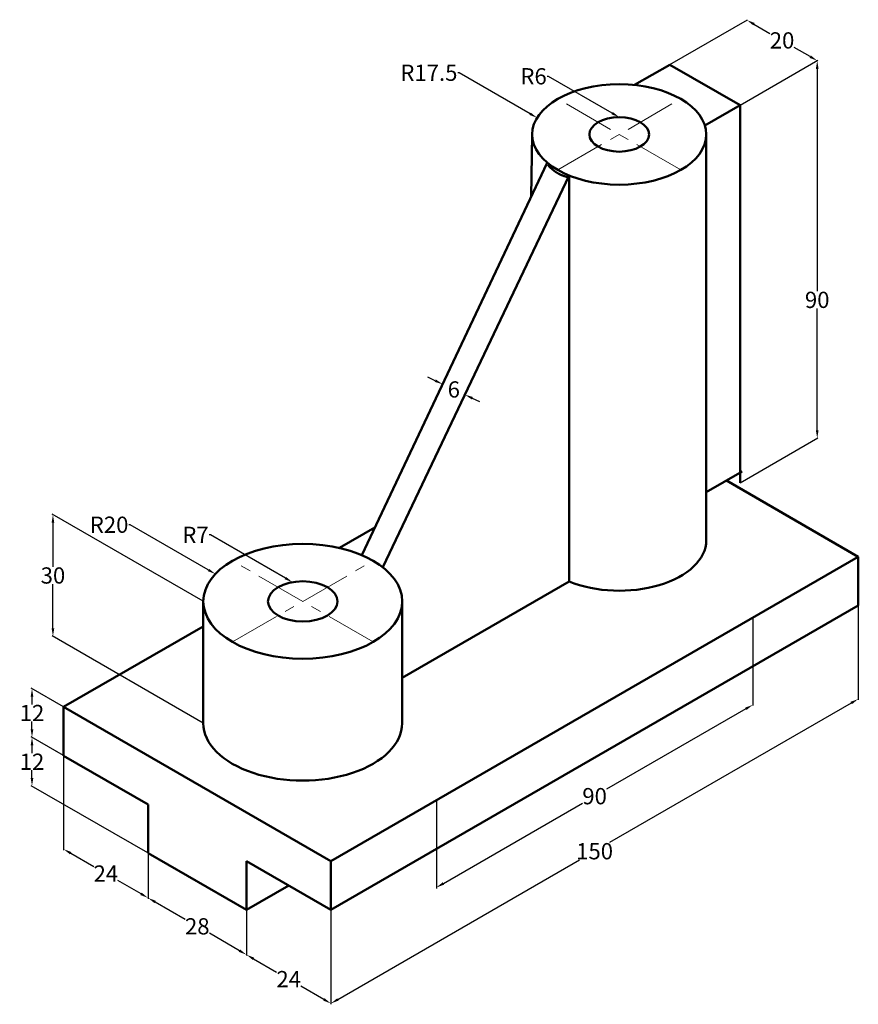
# Model space of a CAD drawing. Units: millimetres. Extents: x -18 to 188, y -21 to 222.
import ezdxf
from ezdxf import colors
from ezdxf.entities.mleader import LeaderData, LeaderLine
from ezdxf.math import Vec2, Vec3

# ---------------------------------------------------------------- set-up
doc = ezdxf.new("R2010")
doc.units = ezdxf.units.MM
doc.header["$MEASUREMENT"] = 0
doc.linetypes.add('CENTER', pattern=[2, 1.25, -0.25, 0.25, -0.25])
for name, color, linetype, lineweight in [('M-CNTR', 1, 'CENTER', 18), ('M-DIMS', 2, 'Continuous', 25), ('M-OUTL', 7, 'Continuous', 50)]:
    doc.layers.add(name, color=color, linetype=linetype, lineweight=lineweight)
doc.styles.get("Standard").update_dxf_attribs({"font": 'arial.ttf'})
doc.dimstyles.get("Standard").update_dxf_attribs({"dimtxt": 4, "dimasz": 2, "dimexe": 0.18, "dimexo": 0.0625, "dimgap": 0.09, "dimtad": 0, "dimtih": 1, "dimtoh": 1, "dimdec": 0, "dimzin": 0, "dimdsep": 46, "dimtxsty": 'Standard', "dimcen": 0.09, "dimadec": 0, "dimazin": 0, "dimtfac": 1, "dimtdec": 0, "dimtofl": 0, "dimtmove": 0, "dimatfit": 3, "dimfxl": 1, "dimtolj": 1, "dimtzin": 0, "dimarcsym": 0})

# ---------------------------------------------------------------- blocks, each defined once
blk = doc.blocks.new('*D1')
at = {"layer": 'Defpoints', "color": 0, "transparency": 16777216}
for p in [(162.15, 74.6), (162.15, 53.13), (84.21, 29.6)]:
    blk.add_point(p, dxfattribs=at)
at = {"layer": 'M-DIMS', "color": 0, "lineweight": -2, "transparency": 16777216}
for p, q in [((162.15, 74.53), (162.15, 52.92)), ((160.42, 52.13), (126.13, 32.33)), ((84.21, 29.53), (84.21, 7.92)), ((85.94, 9.13), (120.23, 28.93))]:
    blk.add_line(p, q, dxfattribs=at)
at = {"layer": 'M-DIMS', "color": 0, "transparency": 16777216}
for points in [[(160.25, 52.42), (160.59, 51.84), (162.15, 53.13)], [(85.77, 9.42), (86.11, 8.84), (84.21, 8.13)]]:
    blk.add_solid(points, dxfattribs=at)
at = {"layer": 'M-DIMS', "color": 0, "transparency": 16777216, "insert": (123.18, 30.63), "char_height": 4, "attachment_point": 5}
blk.add_mtext('\\A1;90', dxfattribs=at)
blk = doc.blocks.new('*D2')
at = {"layer": 'Defpoints', "color": 0, "transparency": 16777216}
for p in [(188.13, 77.6), (58.23, 2.6), (58.23, -20.43)]:
    blk.add_point(p, dxfattribs=at)
at = {"layer": 'M-DIMS', "color": 0, "lineweight": -2, "transparency": 16777216}
for p, q in [((188.13, 77.53), (188.13, 54.37)), ((186.4, 53.57), (126.87, 19.21)), ((59.96, -19.43), (119.49, 14.94)), ((58.23, 2.53), (58.23, -20.63))]:
    blk.add_line(p, q, dxfattribs=at)
at = {"layer": 'M-DIMS', "color": 0, "transparency": 16777216}
for points in [[(186.23, 53.86), (186.57, 53.29), (188.13, 54.57)], [(59.79, -19.14), (60.13, -19.71), (58.23, -20.43)]]:
    blk.add_solid(points, dxfattribs=at)
at = {"layer": 'M-DIMS', "color": 0, "transparency": 16777216, "insert": (123.18, 17.07), "char_height": 4, "attachment_point": 5}
blk.add_mtext('\\A1;150', dxfattribs=at)
blk = doc.blocks.new('*D3')
at = {"layer": 'Defpoints', "color": 0, "transparency": 16777216}
for p in [(37.44, 14.6), (58.23, 2.6), (58.23, -20.43)]:
    blk.add_point(p, dxfattribs=at)
at = {"layer": 'M-DIMS', "color": 0, "lineweight": -2, "transparency": 16777216}
for p, q in [((37.44, 14.53), (37.44, -8.63)), ((58.23, 2.53), (58.23, -20.63)), ((39.18, -9.43), (44.86, -12.7)), ((56.5, -19.43), (50.82, -16.15))]:
    blk.add_line(p, q, dxfattribs=at)
at = {"layer": 'M-DIMS', "color": 0, "transparency": 16777216}
for points in [[(39.34, -9.14), (39.01, -9.71), (37.44, -8.43)], [(56.66, -19.14), (56.33, -19.71), (58.23, -20.43)]]:
    blk.add_solid(points, dxfattribs=at)
at = {"layer": 'M-DIMS', "color": 0, "transparency": 16777216, "insert": (47.84, -14.43), "char_height": 4, "attachment_point": 5}
blk.add_mtext('\\A1;24', dxfattribs=at)
blk = doc.blocks.new('*D4')
at = {"layer": 'Defpoints', "color": 0, "transparency": 16777216}
for p in [(13.19, 16.6), (13.19, 5.57), (37.44, 2.6)]:
    blk.add_point(p, dxfattribs=at)
at = {"layer": 'M-DIMS', "color": 0, "lineweight": -2, "transparency": 16777216}
for p, q in [((13.19, 16.53), (13.19, 5.37)), ((14.93, 4.57), (22.33, 0.3)), ((37.44, 2.53), (37.44, -8.63)), ((35.71, -7.43), (28.31, -3.15))]:
    blk.add_line(p, q, dxfattribs=at)
at = {"layer": 'M-DIMS', "color": 0, "transparency": 16777216}
for points in [[(15.09, 4.86), (14.76, 4.29), (13.19, 5.57)], [(35.88, -7.14), (35.54, -7.71), (37.44, -8.43)]]:
    blk.add_solid(points, dxfattribs=at)
at = {"layer": 'M-DIMS', "color": 0, "transparency": 16777216, "insert": (25.32, -1.43), "char_height": 4, "attachment_point": 5}
blk.add_mtext('\\A1;28', dxfattribs=at)
blk = doc.blocks.new('*D5')
at = {"layer": 'Defpoints', "color": 0, "transparency": 16777216}
for p in [(-7.59, 40.6), (13.19, 28.6), (-7.59, 17.57)]:
    blk.add_point(p, dxfattribs=at)
at = {"layer": 'M-DIMS', "color": 0, "lineweight": -2, "transparency": 16777216}
for p, q in [((-7.59, 40.53), (-7.59, 17.37)), ((13.19, 28.53), (13.19, 5.37)), ((-5.86, 16.57), (-0.18, 13.3)), ((11.46, 6.57), (5.78, 9.85))]:
    blk.add_line(p, q, dxfattribs=at)
at = {"layer": 'M-DIMS', "color": 0, "transparency": 16777216}
for points in [[(-5.69, 16.86), (-6.02, 16.29), (-7.59, 17.57)], [(11.63, 6.86), (11.3, 6.29), (13.19, 5.57)]]:
    blk.add_solid(points, dxfattribs=at)
at = {"layer": 'M-DIMS', "color": 0, "transparency": 16777216, "insert": (2.8, 11.57), "char_height": 4, "attachment_point": 5}
blk.add_mtext('\\A1;24', dxfattribs=at)
blk = doc.blocks.new('*D6')
at = {"layer": 'Defpoints', "color": 0, "transparency": 16777216}
for p in [(-15.39, 57.11), (-7.59, 52.6), (-7.59, 40.6)]:
    blk.add_point(p, dxfattribs=at)
at = {"layer": 'M-DIMS', "color": 0, "lineweight": -2, "transparency": 16777216}
for p, q in [((-7.65, 52.64), (-15.57, 57.21)), ((-15.39, 55.11), (-15.39, 53.21)), ((-15.39, 47.11), (-15.39, 49.01)), ((-7.65, 40.64), (-15.57, 45.21))]:
    blk.add_line(p, q, dxfattribs=at)
at = {"layer": 'M-DIMS', "color": 0, "transparency": 16777216}
for points in [[(-15.72, 55.11), (-15.06, 55.11), (-15.39, 57.11)], [(-15.72, 47.11), (-15.06, 47.11), (-15.39, 45.11)]]:
    blk.add_solid(points, dxfattribs=at)
at = {"layer": 'M-DIMS', "color": 0, "transparency": 16777216, "insert": (-15.39, 51.11), "char_height": 4, "attachment_point": 5}
blk.add_mtext('\\A1;12', dxfattribs=at)
blk = doc.blocks.new('*D7')
at = {"layer": 'Defpoints', "color": 0, "transparency": 16777216}
for p in [(-15.39, 45.11), (13.19, 28.6), (13.19, 16.6)]:
    blk.add_point(p, dxfattribs=at)
at = {"layer": 'M-DIMS', "color": 0, "lineweight": -2, "transparency": 16777216}
for p, q in [((13.13, 28.64), (-15.57, 45.21)), ((-15.39, 43.11), (-15.39, 41.21)), ((-15.39, 35.11), (-15.39, 37.01)), ((13.13, 16.64), (-15.57, 33.21))]:
    blk.add_line(p, q, dxfattribs=at)
at = {"layer": 'M-DIMS', "color": 0, "transparency": 16777216}
for points in [[(-15.72, 43.11), (-15.06, 43.11), (-15.39, 45.11)], [(-15.72, 35.11), (-15.06, 35.11), (-15.39, 33.11)]]:
    blk.add_solid(points, dxfattribs=at)
at = {"layer": 'M-DIMS', "color": 0, "transparency": 16777216, "insert": (-15.39, 39.11), "char_height": 4, "attachment_point": 5}
blk.add_mtext('\\A1;12', dxfattribs=at)
blk = doc.blocks.new('*D8')
at = {"layer": 'Defpoints', "color": 0, "transparency": 16777216}
for p in [(-10.23, 99.98), (26.81, 78.6), (26.81, 48.6)]:
    blk.add_point(p, dxfattribs=at)
at = {"layer": 'M-DIMS', "color": 0, "lineweight": -2, "transparency": 16777216}
for p, q in [((26.74, 78.64), (-10.41, 100.09)), ((-10.23, 97.98), (-10.23, 87.12)), ((-10.23, 71.98), (-10.23, 82.85)), ((26.74, 48.64), (-10.41, 70.09))]:
    blk.add_line(p, q, dxfattribs=at)
at = {"layer": 'M-DIMS', "color": 0, "transparency": 16777216}
for points in [[(-10.56, 97.98), (-9.9, 97.98), (-10.23, 99.98)], [(-10.56, 71.98), (-9.9, 71.98), (-10.23, 69.98)]]:
    blk.add_solid(points, dxfattribs=at)
at = {"layer": 'M-DIMS', "color": 0, "transparency": 16777216, "insert": (-10.23, 84.98), "char_height": 4, "attachment_point": 5}
blk.add_mtext('\\A1;30', dxfattribs=at)
blk = doc.blocks.new('*D9')
at = {"layer": 'Defpoints', "color": 0, "transparency": 16777216}
for p in [(88.46, 137.84), (93.97, 135.24), (85.74, 132.1)]:
    blk.add_point(p, dxfattribs=at)
at = {"layer": 'M-DIMS', "color": 0, "lineweight": -2, "transparency": 16777216}
for p, q in [((88.43, 137.79), (85.67, 131.94)), ((83.93, 132.96), (82.13, 133.81)), ((93.94, 135.18), (91.18, 129.34)), ((93.06, 128.64), (94.87, 127.79))]:
    blk.add_line(p, q, dxfattribs=at)
at = {"layer": 'M-DIMS', "color": 0, "transparency": 16777216}
for points in [[(84.08, 133.26), (83.79, 132.66), (85.74, 132.1)], [(93.2, 128.95), (92.92, 128.34), (91.25, 129.5)]]:
    blk.add_solid(points, dxfattribs=at)
at = {"layer": 'M-DIMS', "color": 0, "transparency": 16777216, "insert": (88.5, 130.8), "char_height": 4, "attachment_point": 5}
blk.add_mtext('\\A1;6', dxfattribs=at)
blk = doc.blocks.new('*D10')
at = {"layer": 'Defpoints', "color": 0, "transparency": 16777216}
for p in [(178.01, 211.76), (141.68, 210.78), (159, 200.78)]:
    blk.add_point(p, dxfattribs=at)
at = {"layer": 'M-DIMS', "color": 0, "lineweight": -2, "transparency": 16777216}
for p, q in [((141.74, 210.82), (160.87, 221.86)), ((162.42, 220.76), (166.37, 218.48)), ((176.28, 212.76), (172.33, 215.04)), ((159.06, 200.82), (178.19, 211.86))]:
    blk.add_line(p, q, dxfattribs=at)
at = {"layer": 'M-DIMS', "color": 0, "transparency": 16777216}
for points in [[(162.59, 221.05), (162.26, 220.47), (160.69, 221.76)], [(176.45, 213.05), (176.11, 212.47), (178.01, 211.76)]]:
    blk.add_solid(points, dxfattribs=at)
at = {"layer": 'M-DIMS', "color": 0, "transparency": 16777216, "insert": (169.35, 216.76), "char_height": 4, "attachment_point": 5}
blk.add_mtext('\\A1;20', dxfattribs=at)
blk = doc.blocks.new('*D11')
at = {"layer": 'Defpoints', "color": 0, "transparency": 16777216}
for p in [(178.01, 211.76), (159, 200.78), (159, 107.78)]:
    blk.add_point(p, dxfattribs=at)
at = {"layer": 'M-DIMS', "color": 0, "lineweight": -2, "transparency": 16777216}
for p, q in [((159.06, 200.82), (178.19, 211.86)), ((178.01, 209.76), (178.01, 154.99)), ((178.01, 120.76), (178.01, 150.73)), ((159.06, 107.82), (178.19, 118.86))]:
    blk.add_line(p, q, dxfattribs=at)
at = {"layer": 'M-DIMS', "color": 0, "transparency": 16777216}
for points in [[(177.68, 209.76), (178.34, 209.76), (178.01, 211.76)], [(177.68, 120.76), (178.34, 120.76), (178.01, 118.76)]]:
    blk.add_solid(points, dxfattribs=at)
at = {"layer": 'M-DIMS', "color": 0, "transparency": 16777216, "insert": (178.01, 152.86), "char_height": 4, "attachment_point": 5}
blk.add_mtext('\\A1;90', dxfattribs=at)

msp = doc.modelspace()

# ---------------------------------------------------------------- linework, layer by layer
at = {"layer": 'M-CNTR', "ltscale": 10}
for p, q in [((114.09, 184.85), (144.4, 202.35)), ((144.4, 184.85), (114.09, 202.35)), ((68.62, 68.6), (33.98, 88.6)), ((33.98, 68.6), (68.62, 88.6))]:
    msp.add_line(p, q, dxfattribs=at)
at = {"layer": 'M-OUTL'}
for p, q in [((133.02, 205.78), (141.68, 210.78)), ((141.68, 210.78), (159, 200.78)), ((159, 200.78), (150.34, 195.78)), ((159, 200.78), (159, 107.78)), ((107.81, 193.6), (107.57, 178.27)), ((150.68, 193.6), (150.68, 93.6)), ((111.53, 186.64), (65.83, 89.99)), ((116.91, 183.48), (71.02, 86.99)), ((116.91, 183.48), (116.91, 83.48)), ((60.33, 91.75), (69.03, 96.77)), ((58.23, 14.6), (188.13, 89.6)), ((188.13, 89.6), (188.13, 77.6)), ((116.91, 83.48), (75.79, 59.74)), ((26.81, 78.6), (26.81, 48.6)), ((188.13, 77.6), (58.23, 2.6)), ((75.79, 78.6), (75.79, 48.6)), ((-7.59, 52.6), (26.81, 72.39)), ((18.44, 67.58), (18.39, 67.6)), ((-7.59, 40.6), (-7.59, 52.6)), ((58.23, 14.6), (-7.59, 52.6)), ((13.19, 28.6), (-7.59, 40.6)), ((13.19, 16.6), (13.19, 28.6)), ((37.44, 2.6), (13.19, 16.6)), ((58.23, 2.6), (37.44, 14.6)), ((37.44, 14.6), (37.44, 2.6)), ((58.23, 2.6), (58.23, 14.6))]:
    msp.add_line(p, q, dxfattribs=at)
at = {"layer": 'M-OUTL', "ltscale": 100}
for p, q in [((150.68, 105.48), (159.55, 110.6)), ((188.13, 89.6), (155.66, 108.35)), ((37.44, 2.6), (47.84, 8.6))]:
    msp.add_line(p, q, dxfattribs=at)
msp.add_lwpolyline([(116.91, 183.03), (116.85, 183.04), (116.78, 183.06), (116.72, 183.07), (116.66, 183.08), (116.6, 183.09), (116.54, 183.11), (116.47, 183.12), (116.41, 183.14), (116.35, 183.15), (116.29, 183.17), (116.23, 183.18), (116.17, 183.2), (116.11, 183.21), (116.04, 183.23), (115.98, 183.25), (115.92, 183.27), (115.86, 183.29), (115.8, 183.3), (115.74, 183.32), (115.68, 183.34), (115.62, 183.36), (115.57, 183.38), (115.51, 183.4), (115.45, 183.43), (115.39, 183.45), (115.33, 183.47), (115.27, 183.49), (115.21, 183.51), (115.16, 183.54), (115.1, 183.56), (115.04, 183.59), (114.98, 183.61), (114.92, 183.63), (114.87, 183.66), (114.81, 183.68), (114.75, 183.71), (114.7, 183.74), (114.64, 183.77), (114.59, 183.79), (114.53, 183.82), (114.47, 183.85), (114.42, 183.88), (114.36, 183.91), (114.31, 183.94), (114.25, 183.97), (114.2, 184), (114.14, 184.03), (114.09, 184.06), (114.03, 184.09), (113.98, 184.12), (113.93, 184.16), (113.87, 184.19), (113.82, 184.22), (113.76, 184.25), (113.71, 184.29), (113.66, 184.32), (113.61, 184.36), (113.55, 184.39), (113.5, 184.43), (113.45, 184.47), (113.4, 184.5), (113.34, 184.54), (113.29, 184.58), (113.24, 184.61), (113.19, 184.65), (113.14, 184.69), (113.09, 184.73), (113.04, 184.77), (112.99, 184.81), (112.94, 184.85), (112.89, 184.89), (112.84, 184.93), (112.79, 184.97), (112.74, 185.01), (112.69, 185.05), (112.64, 185.1), (112.6, 185.14), (112.55, 185.18), (112.5, 185.23), (112.45, 185.27), (112.4, 185.32), (112.35, 185.36), (112.31, 185.41), (112.26, 185.45), (112.21, 185.5), (112.17, 185.55), (112.12, 185.59), (112.08, 185.64), (112.03, 185.69), (111.98, 185.73), (111.94, 185.78), (111.89, 185.83), (111.85, 185.88), (111.8, 185.93), (111.76, 185.98), (111.71, 186.03)], dxfattribs=at)
at = {"layer": 'M-OUTL'}
for centre, major_axis in [((129.24, 193.6), (-21.43, 0)), ((129.24, 193.6), (-7.35, 0)), ((51.3, 78.6), (-24.49, 0)), ((51.3, 78.6), (-8.57, 0))]:
    msp.add_ellipse(centre, major_axis=major_axis, ratio=0.57735, dxfattribs=at)
for centre, major_axis, start_param in [((129.24, 93.6), (-21.43, 0), 0.957678), ((51.3, 48.6), (-24.49, 0), 0)]:
    msp.add_ellipse(centre, major_axis=major_axis, ratio=0.57735, start_param=start_param, end_param=3.141593, dxfattribs=at)

# ---------------------------------------------------------------- dimensions: what is measured, and where the dimension line sits
at = {"layer": 'M-DIMS'}
for p1, p2, distance, picture, middle in [((141.68, 210.78), (159, 200.78), 19.01, '*D10', (169.35, 216.76)), ((93.97, 135.24), (88.46, 137.84), 6.35, '*D9', (88.5, 130.8)), ((26.81, 48.6), (26.81, 78.6), 37.03, '*D8', (-10.23, 84.98)), ((188.13, 77.6), (58.23, 2.6), 19.94, '*D2', (123.18, 17.07)), ((84.21, 29.6), (162.15, 74.6), -18.59, '*D1', (123.18, 30.63)), ((-7.59, 40.6), (-7.59, 52.6), 7.8, '*D6', (-15.39, 51.11)), ((13.19, 16.6), (13.19, 28.6), 28.59, '*D7', (-15.39, 39.11)), ((13.19, 28.6), (-7.59, 40.6), 19.94, '*D5', (2.8, 11.57)), ((37.44, 2.6), (13.19, 16.6), 9.55, '*D4', (25.32, -1.43)), ((37.44, 14.6), (58.23, 2.6), -19.94, '*D3', (47.84, -14.43))]:
    dim = msp.add_aligned_dim(p1=p1, p2=p2, distance=distance, dimstyle='Standard', override={"dimclrd": 0, "dimclre": 0, "dimclrt": 0}, dxfattribs=at)
    dim.commit()
    dim.dimension.update_dxf_attribs({"geometry": picture, "text_midpoint": middle})
dim = msp.add_linear_dim(base=(178.01, 211.76), p1=(159, 107.78), p2=(159, 200.78), angle=90, text='90', dimstyle='Standard', override={"dimclrd": 0, "dimclre": 0, "dimclrt": 0}, dxfattribs=at)
dim.commit()
dim.dimension.update_dxf_attribs({"geometry": '*D11', "text_midpoint": (178.01, 152.86), "dimtype": 161})

# ---------------------------------------------------------------- leaders
ml = msp.add_multileader_mtext('Standard', dxfattribs=at)
ml.set_content('R17.5', color=256)
ml.set_leader_properties()
ml.build(insert=Vec2(0, 0))
ml.multileader.update_dxf_attribs({"dogleg_length": 0.36, "arrow_head_size": 2})
ctx = ml.context
ctx.base_point, ctx.arrow_head_size, ctx.landing_gap_size, ctx.plane_origin = Vec3(75.06, 208.77), 2, 0.09, Vec3(109.02, 197.7)
ctx.text_align_type = 2
notes = []
notes.append((ctx, [(0, (1, 1, 0), (89.85, 208.77), (-1, 0), 0.36, [(0, [(109.02, 197.7)], 0, [])])]))
ctx.mtext.insert, ctx.mtext.alignment, ctx.mtext.flow_direction = Vec3(89.4, 210.8), 3, 5
ml = msp.add_multileader_mtext('Standard', dxfattribs=at)
ml.set_content('R6', color=256)
ml.set_leader_properties()
ml.build(insert=Vec2(0, 0))
ml.multileader.update_dxf_attribs({"dogleg_length": 0.36, "arrow_head_size": 2})
ctx = ml.context
ctx.base_point, ctx.arrow_head_size, ctx.landing_gap_size, ctx.plane_origin = Vec3(104.85, 207.89), 2, 0.09, Vec3(129.24, 197.85)
ctx.text_align_type = 2
notes.append((ctx, [(0, (1, 1, 0), (111.84, 207.89), (-1, 0), 0.36, [(0, [(129.24, 197.85)], 0, [])])]))
ctx.mtext.insert, ctx.mtext.alignment, ctx.mtext.flow_direction = Vec3(111.39, 209.93), 3, 5
ml = msp.add_multileader_mtext('Standard', dxfattribs=at)
ml.set_content('R20', color=256)
ml.set_leader_properties()
ml.build(insert=Vec2(0, 0))
ml.multileader.update_dxf_attribs({"dogleg_length": 0.36, "arrow_head_size": 2})
ctx = ml.context
ctx.base_point, ctx.arrow_head_size, ctx.landing_gap_size, ctx.plane_origin = Vec3(-1.28, 97.45), 2, 0.09, Vec3(29.77, 85.35)
ctx.text_align_type = 2
notes.append((ctx, [(0, (1, 1, 0), (8.81, 97.45), (-1, 0), 0.36, [(0, [(29.77, 85.35)], 0, [])])]))
ctx.mtext.insert, ctx.mtext.alignment, ctx.mtext.flow_direction = Vec3(8.36, 99.48), 3, 5
ml = msp.add_multileader_mtext('Standard', dxfattribs=at)
ml.set_content('R7', color=256)
ml.set_leader_properties()
ml.build(insert=Vec2(0, 0))
ml.multileader.update_dxf_attribs({"dogleg_length": 0.36, "arrow_head_size": 2})
ctx = ml.context
ctx.base_point, ctx.arrow_head_size, ctx.landing_gap_size, ctx.plane_origin = Vec3(21.58, 94.99), 2, 0.09, Vec3(48.76, 83.33)
ctx.text_align_type = 2
notes.append((ctx, [(0, (1, 1, 0), (28.57, 94.99), (-1, 0), 0.36, [(0, [(48.76, 83.33)], 0, [])])]))
ctx.mtext.insert, ctx.mtext.alignment, ctx.mtext.flow_direction = Vec3(28.12, 96.99), 3, 5
for ctx, leaders in notes:
    for number, flags, end, landing, length, lines in leaders:
        leader = LeaderData()
        leader.index, (leader.has_last_leader_line, leader.has_dogleg_vector, leader.attachment_direction) = number, flags
        leader.last_leader_point, leader.dogleg_vector, leader.dogleg_length = Vec3(end), Vec3(landing), length
        for number, points, colour, breaks in lines:
            line = LeaderLine()
            line.index, line.vertices, line.color, line.breaks = number, Vec3.list(points), colors.encode_raw_color(colour), breaks
            leader.lines.append(line)
        ctx.leaders.append(leader)

doc.saveas('drawing.dxf')
